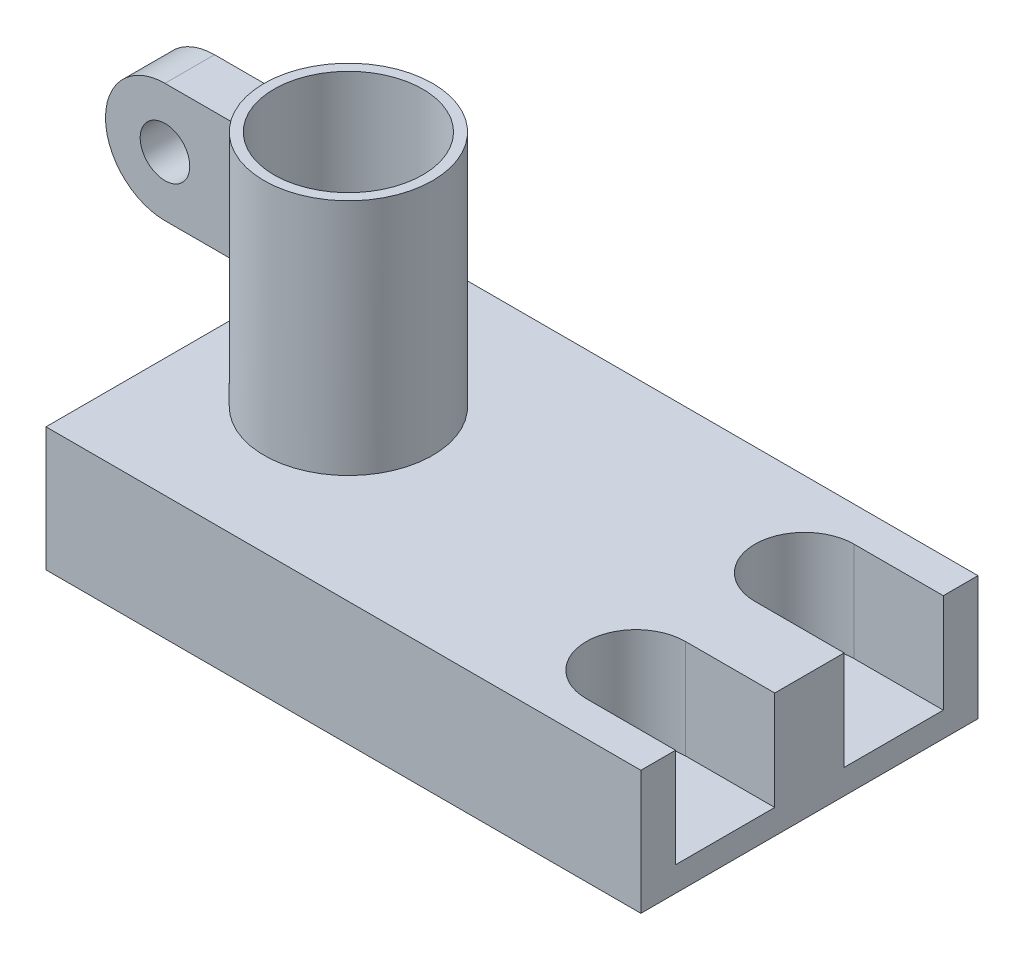
ISO-10303-21;
HEADER;
FILE_DESCRIPTION(('STEP AP214'),'2;1');
FILE_NAME('part.step','',(''),(''),'','','');
FILE_SCHEMA(('AUTOMOTIVE_DESIGN { 1 0 10303 214 1 1 1 1 }'));
ENDSEC;
DATA;
#1=APPLICATION_CONTEXT('core data for automotive mechanical design processes');
#2=APPLICATION_PROTOCOL_DEFINITION('international standard','automotive_design',2000,#1);
#3=PRODUCT_CONTEXT('',#1,'mechanical');
#4=PRODUCT('Part','Part','',(#3));
#5=PRODUCT_RELATED_PRODUCT_CATEGORY('part','',(#4));
#6=PRODUCT_DEFINITION_FORMATION('','',#4);
#7=PRODUCT_DEFINITION_CONTEXT('part definition',#1,'design');
#8=PRODUCT_DEFINITION('design','',#6,#7);
#9=PRODUCT_DEFINITION_SHAPE('','',#8);
#10=(LENGTH_UNIT() NAMED_UNIT(*) SI_UNIT(.MILLI.,.METRE.));
#11=(NAMED_UNIT(*) PLANE_ANGLE_UNIT() SI_UNIT($,.RADIAN.));
#12=(NAMED_UNIT(*) SI_UNIT($,.STERADIAN.) SOLID_ANGLE_UNIT());
#13=UNCERTAINTY_MEASURE_WITH_UNIT(LENGTH_MEASURE(1.E-05),#10,'distance_accuracy_value','');
#14=(GEOMETRIC_REPRESENTATION_CONTEXT(3) GLOBAL_UNCERTAINTY_ASSIGNED_CONTEXT((#13)) GLOBAL_UNIT_ASSIGNED_CONTEXT((#10,
#11,#12)) REPRESENTATION_CONTEXT('',''));
#15=CARTESIAN_POINT('',(0.,0.,0.));
#16=DIRECTION('',(0.,0.,1.));
#17=DIRECTION('',(1.,0.,0.));
#18=AXIS2_PLACEMENT_3D('',#15,#16,#17);
#19=CARTESIAN_POINT('',(60.,25.,34.));
#20=DIRECTION('',(-1.,0.,0.));
#21=DIRECTION('',(0.,0.,1.));
#22=AXIS2_PLACEMENT_3D('',#19,#20,#21);
#23=PLANE('',#22);
#24=DIRECTION('',(0.,0.,-1.));
#25=VECTOR('',#24,1.);
#26=CARTESIAN_POINT('',(60.,25.,34.));
#27=LINE('',#26,#25);
#28=CARTESIAN_POINT('',(60.,25.,-27.));
#29=VERTEX_POINT('',#28);
#30=CARTESIAN_POINT('',(60.,25.,-34.));
#31=VERTEX_POINT('',#30);
#32=EDGE_CURVE('E275',#29,#31,#27,.T.);
#33=ORIENTED_EDGE('',*,*,#32,.F.);
#34=DIRECTION('',(0.,1.,0.));
#35=VECTOR('',#34,1.);
#36=CARTESIAN_POINT('',(60.,5.,-27.));
#37=LINE('',#36,#35);
#38=CARTESIAN_POINT('',(60.,5.,-27.));
#39=VERTEX_POINT('',#38);
#40=EDGE_CURVE('E194',#39,#29,#37,.T.);
#41=ORIENTED_EDGE('',*,*,#40,.F.);
#42=DIRECTION('',(0.,0.,-1.));
#43=VECTOR('',#42,1.);
#44=CARTESIAN_POINT('',(60.,5.,-27.));
#45=LINE('',#44,#43);
#46=CARTESIAN_POINT('',(60.,5.,-6.99999999999999));
#47=VERTEX_POINT('',#46);
#48=EDGE_CURVE('E175',#47,#39,#45,.T.);
#49=ORIENTED_EDGE('',*,*,#48,.F.);
#50=DIRECTION('',(0.,1.,0.));
#51=VECTOR('',#50,1.);
#52=CARTESIAN_POINT('',(60.,5.,-6.99999999999999));
#53=LINE('',#52,#51);
#54=CARTESIAN_POINT('',(60.,25.,-6.99999999999999));
#55=VERTEX_POINT('',#54);
#56=EDGE_CURVE('E161',#47,#55,#53,.T.);
#57=ORIENTED_EDGE('',*,*,#56,.T.);
#58=CARTESIAN_POINT('',(60.,25.,7.00000000000001));
#59=VERTEX_POINT('',#58);
#60=EDGE_CURVE('E272',#59,#55,#27,.T.);
#61=ORIENTED_EDGE('',*,*,#60,.F.);
#62=DIRECTION('',(0.,1.,0.));
#63=VECTOR('',#62,1.);
#64=CARTESIAN_POINT('',(60.,5.,7.00000000000001));
#65=LINE('',#64,#63);
#66=CARTESIAN_POINT('',(60.,5.,7.00000000000001));
#67=VERTEX_POINT('',#66);
#68=EDGE_CURVE('E213',#67,#59,#65,.T.);
#69=ORIENTED_EDGE('',*,*,#68,.F.);
#70=DIRECTION('',(0.,0.,-1.));
#71=VECTOR('',#70,1.);
#72=CARTESIAN_POINT('',(60.,5.,7.00000000000001));
#73=LINE('',#72,#71);
#74=CARTESIAN_POINT('',(60.,5.,27.));
#75=VERTEX_POINT('',#74);
#76=EDGE_CURVE('E201',#75,#67,#73,.T.);
#77=ORIENTED_EDGE('',*,*,#76,.F.);
#78=DIRECTION('',(0.,1.,0.));
#79=VECTOR('',#78,1.);
#80=CARTESIAN_POINT('',(60.,5.,27.));
#81=LINE('',#80,#79);
#82=CARTESIAN_POINT('',(60.,25.,27.));
#83=VERTEX_POINT('',#82);
#84=EDGE_CURVE('E219',#75,#83,#81,.T.);
#85=ORIENTED_EDGE('',*,*,#84,.T.);
#86=CARTESIAN_POINT('',(60.,25.,34.));
#87=VERTEX_POINT('',#86);
#88=EDGE_CURVE('E270',#87,#83,#27,.T.);
#89=ORIENTED_EDGE('',*,*,#88,.F.);
#90=DIRECTION('',(0.,-1.,0.));
#91=VECTOR('',#90,1.);
#92=CARTESIAN_POINT('',(60.,25.,34.));
#93=LINE('',#92,#91);
#94=CARTESIAN_POINT('',(60.,0.,34.));
#95=VERTEX_POINT('',#94);
#96=EDGE_CURVE('E279',#87,#95,#93,.T.);
#97=ORIENTED_EDGE('',*,*,#96,.T.);
#98=DIRECTION('',(0.,0.,-1.));
#99=VECTOR('',#98,1.);
#100=CARTESIAN_POINT('',(60.,0.,34.));
#101=LINE('',#100,#99);
#102=CARTESIAN_POINT('',(60.,0.,-34.));
#103=VERTEX_POINT('',#102);
#104=EDGE_CURVE('E268',#95,#103,#101,.T.);
#105=ORIENTED_EDGE('',*,*,#104,.T.);
#106=DIRECTION('',(0.,-1.,0.));
#107=VECTOR('',#106,1.);
#108=CARTESIAN_POINT('',(60.,25.,-34.));
#109=LINE('',#108,#107);
#110=EDGE_CURVE('E294',#31,#103,#109,.T.);
#111=ORIENTED_EDGE('',*,*,#110,.F.);
#112=EDGE_LOOP('',(#33,#41,#49,#57,#61,#69,#77,#85,#89,#97,#105,#111));
#113=FACE_BOUND('',#112,.T.);
#114=ADVANCED_FACE('F44',(#113),#23,.F.);
#115=CARTESIAN_POINT('',(-60.,25.,-34.));
#116=DIRECTION('',(0.,0.,1.));
#117=DIRECTION('',(1.,0.,0.));
#118=AXIS2_PLACEMENT_3D('',#115,#116,#117);
#119=PLANE('',#118);
#120=DIRECTION('',(-1.,0.,0.));
#121=VECTOR('',#120,1.);
#122=CARTESIAN_POINT('',(-60.,0.,-34.));
#123=LINE('',#122,#121);
#124=CARTESIAN_POINT('',(-60.,0.,-34.));
#125=VERTEX_POINT('',#124);
#126=EDGE_CURVE('E283',#103,#125,#123,.T.);
#127=ORIENTED_EDGE('',*,*,#126,.T.);
#128=DIRECTION('',(0.,-1.,0.));
#129=VECTOR('',#128,1.);
#130=CARTESIAN_POINT('',(-60.,25.,-34.));
#131=LINE('',#130,#129);
#132=CARTESIAN_POINT('',(-60.,25.,-34.));
#133=VERTEX_POINT('',#132);
#134=EDGE_CURVE('E292',#133,#125,#131,.T.);
#135=ORIENTED_EDGE('',*,*,#134,.F.);
#136=DIRECTION('',(-1.,0.,0.));
#137=VECTOR('',#136,1.);
#138=CARTESIAN_POINT('',(-60.,25.,-34.));
#139=LINE('',#138,#137);
#140=EDGE_CURVE('E267',#31,#133,#139,.T.);
#141=ORIENTED_EDGE('',*,*,#140,.F.);
#142=ORIENTED_EDGE('',*,*,#110,.T.);
#143=EDGE_LOOP('',(#127,#135,#141,#142));
#144=FACE_BOUND('',#143,.T.);
#145=ADVANCED_FACE('F345',(#144),#119,.F.);
#146=CARTESIAN_POINT('',(-60.,25.,34.));
#147=DIRECTION('',(1.,0.,0.));
#148=DIRECTION('',(0.,0.,-1.));
#149=AXIS2_PLACEMENT_3D('',#146,#147,#148);
#150=PLANE('',#149);
#151=DIRECTION('',(0.,0.,1.));
#152=VECTOR('',#151,1.);
#153=CARTESIAN_POINT('',(-60.,0.,34.));
#154=LINE('',#153,#152);
#155=CARTESIAN_POINT('',(-60.,0.,34.));
#156=VERTEX_POINT('',#155);
#157=EDGE_CURVE('E282',#125,#156,#154,.T.);
#158=ORIENTED_EDGE('',*,*,#157,.T.);
#159=DIRECTION('',(0.,-1.,0.));
#160=VECTOR('',#159,1.);
#161=CARTESIAN_POINT('',(-60.,25.,34.));
#162=LINE('',#161,#160);
#163=CARTESIAN_POINT('',(-60.,25.,34.));
#164=VERTEX_POINT('',#163);
#165=EDGE_CURVE('E289',#164,#156,#162,.T.);
#166=ORIENTED_EDGE('',*,*,#165,.F.);
#167=DIRECTION('',(0.,0.,1.));
#168=VECTOR('',#167,1.);
#169=CARTESIAN_POINT('',(-60.,25.,34.));
#170=LINE('',#169,#168);
#171=EDGE_CURVE('E274',#133,#164,#170,.T.);
#172=ORIENTED_EDGE('',*,*,#171,.F.);
#173=ORIENTED_EDGE('',*,*,#134,.T.);
#174=EDGE_LOOP('',(#158,#166,#172,#173));
#175=FACE_BOUND('',#174,.T.);
#176=ADVANCED_FACE('F350',(#175),#150,.F.);
#177=CARTESIAN_POINT('',(-60.,25.,34.));
#178=DIRECTION('',(0.,0.,-1.));
#179=DIRECTION('',(-1.,0.,0.));
#180=AXIS2_PLACEMENT_3D('',#177,#178,#179);
#181=PLANE('',#180);
#182=DIRECTION('',(1.,0.,0.));
#183=VECTOR('',#182,1.);
#184=CARTESIAN_POINT('',(-60.,0.,34.));
#185=LINE('',#184,#183);
#186=EDGE_CURVE('E281',#156,#95,#185,.T.);
#187=ORIENTED_EDGE('',*,*,#186,.T.);
#188=ORIENTED_EDGE('',*,*,#96,.F.);
#189=DIRECTION('',(1.,0.,0.));
#190=VECTOR('',#189,1.);
#191=CARTESIAN_POINT('',(-60.,25.,34.));
#192=LINE('',#191,#190);
#193=EDGE_CURVE('E277',#164,#87,#192,.T.);
#194=ORIENTED_EDGE('',*,*,#193,.F.);
#195=ORIENTED_EDGE('',*,*,#165,.T.);
#196=EDGE_LOOP('',(#187,#188,#194,#195));
#197=FACE_BOUND('',#196,.T.);
#198=ADVANCED_FACE('F431',(#197),#181,.F.);
#199=CARTESIAN_POINT('',(0.,25.,0.));
#200=DIRECTION('',(0.,-1.,0.));
#201=DIRECTION('',(0.,0.,-1.));
#202=AXIS2_PLACEMENT_3D('',#199,#200,#201);
#203=PLANE('',#202);
#204=CARTESIAN_POINT('',(-33.,25.,0.));
#205=DIRECTION('',(0.,-1.,0.));
#206=DIRECTION('',(0.,0.,-1.));
#207=AXIS2_PLACEMENT_3D('',#204,#205,#206);
#208=CIRCLE('',#207,17.);
#209=CARTESIAN_POINT('',(-33.,25.,-17.));
#210=VERTEX_POINT('',#209);
#211=EDGE_CURVE('E296',#210,#210,#208,.F.);
#212=ORIENTED_EDGE('',*,*,#211,.F.);
#213=EDGE_LOOP('',(#212));
#214=FACE_BOUND('',#213,.T.);
#215=CARTESIAN_POINT('',(42.,25.,-17.));
#216=DIRECTION('',(0.,1.,0.));
#217=DIRECTION('',(0.,0.,1.));
#218=AXIS2_PLACEMENT_3D('',#215,#216,#217);
#219=CIRCLE('',#218,10.);
#220=CARTESIAN_POINT('',(42.,25.,-27.));
#221=VERTEX_POINT('',#220);
#222=CARTESIAN_POINT('',(42.,25.,-6.99999999999999));
#223=VERTEX_POINT('',#222);
#224=EDGE_CURVE('E58',#221,#223,#219,.T.);
#225=ORIENTED_EDGE('',*,*,#224,.F.);
#226=DIRECTION('',(-1.,0.,0.));
#227=VECTOR('',#226,1.);
#228=CARTESIAN_POINT('',(42.,25.,-27.));
#229=LINE('',#228,#227);
#230=EDGE_CURVE('E176',#29,#221,#229,.T.);
#231=ORIENTED_EDGE('',*,*,#230,.F.);
#232=ORIENTED_EDGE('',*,*,#32,.T.);
#233=ORIENTED_EDGE('',*,*,#140,.T.);
#234=ORIENTED_EDGE('',*,*,#171,.T.);
#235=ORIENTED_EDGE('',*,*,#193,.T.);
#236=ORIENTED_EDGE('',*,*,#88,.T.);
#237=DIRECTION('',(1.,0.,0.));
#238=VECTOR('',#237,1.);
#239=CARTESIAN_POINT('',(60.,25.,27.));
#240=LINE('',#239,#238);
#241=CARTESIAN_POINT('',(42.,25.,27.));
#242=VERTEX_POINT('',#241);
#243=EDGE_CURVE('E208',#242,#83,#240,.T.);
#244=ORIENTED_EDGE('',*,*,#243,.F.);
#245=CARTESIAN_POINT('',(42.,25.,17.));
#246=DIRECTION('',(0.,1.,0.));
#247=DIRECTION('',(0.,0.,1.));
#248=AXIS2_PLACEMENT_3D('',#245,#246,#247);
#249=CIRCLE('',#248,10.);
#250=CARTESIAN_POINT('',(42.,25.,7.00000000000001));
#251=VERTEX_POINT('',#250);
#252=EDGE_CURVE('E67',#251,#242,#249,.T.);
#253=ORIENTED_EDGE('',*,*,#252,.F.);
#254=DIRECTION('',(-1.,0.,0.));
#255=VECTOR('',#254,1.);
#256=CARTESIAN_POINT('',(42.,25.,7.00000000000001));
#257=LINE('',#256,#255);
#258=EDGE_CURVE('E196',#59,#251,#257,.T.);
#259=ORIENTED_EDGE('',*,*,#258,.F.);
#260=ORIENTED_EDGE('',*,*,#60,.T.);
#261=DIRECTION('',(1.,0.,0.));
#262=VECTOR('',#261,1.);
#263=CARTESIAN_POINT('',(60.,25.,-6.99999999999999));
#264=LINE('',#263,#262);
#265=EDGE_CURVE('E177',#223,#55,#264,.T.);
#266=ORIENTED_EDGE('',*,*,#265,.F.);
#267=EDGE_LOOP('',(#225,#231,#232,#233,#234,#235,#236,#244,#253,#259,#260,#266));
#268=FACE_BOUND('',#267,.T.);
#269=ADVANCED_FACE('F359',(#214,#268),#203,.F.);
#270=CARTESIAN_POINT('',(0.,0.,0.));
#271=DIRECTION('',(0.,-1.,0.));
#272=DIRECTION('',(0.,0.,-1.));
#273=AXIS2_PLACEMENT_3D('',#270,#271,#272);
#274=PLANE('',#273);
#275=CARTESIAN_POINT('',(42.,0.,-17.));
#276=DIRECTION('',(0.,-1.,0.));
#277=DIRECTION('',(0.,0.,-1.));
#278=AXIS2_PLACEMENT_3D('',#275,#276,#277);
#279=CIRCLE('',#278,4.00000000000001);
#280=CARTESIAN_POINT('',(42.,0.,-21.));
#281=VERTEX_POINT('',#280);
#282=EDGE_CURVE('E687',#281,#281,#279,.T.);
#283=ORIENTED_EDGE('',*,*,#282,.F.);
#284=EDGE_LOOP('',(#283));
#285=FACE_BOUND('',#284,.T.);
#286=CARTESIAN_POINT('',(42.,0.,17.));
#287=DIRECTION('',(0.,-1.,0.));
#288=DIRECTION('',(0.,0.,-1.));
#289=AXIS2_PLACEMENT_3D('',#286,#287,#288);
#290=CIRCLE('',#289,4.00000000000001);
#291=CARTESIAN_POINT('',(42.,0.,13.));
#292=VERTEX_POINT('',#291);
#293=EDGE_CURVE('E185',#292,#292,#290,.T.);
#294=ORIENTED_EDGE('',*,*,#293,.F.);
#295=EDGE_LOOP('',(#294));
#296=FACE_BOUND('',#295,.T.);
#297=CARTESIAN_POINT('',(-33.,0.,0.));
#298=DIRECTION('',(0.,1.,0.));
#299=DIRECTION('',(0.,0.,1.));
#300=AXIS2_PLACEMENT_3D('',#297,#298,#299);
#301=CIRCLE('',#300,15.);
#302=CARTESIAN_POINT('',(-33.,0.,15.));
#303=VERTEX_POINT('',#302);
#304=EDGE_CURVE('E221',#303,#303,#301,.T.);
#305=ORIENTED_EDGE('',*,*,#304,.T.);
#306=EDGE_LOOP('',(#305));
#307=FACE_BOUND('',#306,.T.);
#308=ORIENTED_EDGE('',*,*,#104,.F.);
#309=ORIENTED_EDGE('',*,*,#186,.F.);
#310=ORIENTED_EDGE('',*,*,#157,.F.);
#311=ORIENTED_EDGE('',*,*,#126,.F.);
#312=EDGE_LOOP('',(#308,#309,#310,#311));
#313=FACE_BOUND('',#312,.T.);
#314=ADVANCED_FACE('F429',(#285,#296,#307,#313),#274,.T.);
#315=CARTESIAN_POINT('',(-33.,73.,0.));
#316=DIRECTION('',(0.,-1.,0.));
#317=DIRECTION('',(0.,0.,-1.));
#318=AXIS2_PLACEMENT_3D('',#315,#316,#317);
#319=CYLINDRICAL_SURFACE('',#318,17.);
#320=CARTESIAN_POINT('',(-33.,68.,0.));
#321=DIRECTION('',(0.,-1.,0.));
#322=DIRECTION('',(0.,0.,-1.));
#323=AXIS2_PLACEMENT_3D('',#320,#321,#322);
#324=CIRCLE('',#323,17.);
#325=CARTESIAN_POINT('',(-49.2480768092719,68.,5.));
#326=VERTEX_POINT('',#325);
#327=CARTESIAN_POINT('',(-49.2480768092719,68.,-5.));
#328=VERTEX_POINT('',#327);
#329=EDGE_CURVE('E302',#326,#328,#324,.T.);
#330=ORIENTED_EDGE('',*,*,#329,.F.);
#331=DIRECTION('',(0.,-1.,0.));
#332=VECTOR('',#331,1.);
#333=CARTESIAN_POINT('',(-49.2480768092719,73.,5.));
#334=LINE('',#333,#332);
#335=CARTESIAN_POINT('',(-49.2480768092719,44.,5.));
#336=VERTEX_POINT('',#335);
#337=EDGE_CURVE('E11',#326,#336,#334,.T.);
#338=ORIENTED_EDGE('',*,*,#337,.T.);
#339=CARTESIAN_POINT('',(-33.,44.,0.));
#340=DIRECTION('',(0.,1.,0.));
#341=DIRECTION('',(0.,0.,1.));
#342=AXIS2_PLACEMENT_3D('',#339,#340,#341);
#343=CIRCLE('',#342,17.);
#344=CARTESIAN_POINT('',(-49.2480768092719,44.,-5.));
#345=VERTEX_POINT('',#344);
#346=EDGE_CURVE('E52',#345,#336,#343,.T.);
#347=ORIENTED_EDGE('',*,*,#346,.F.);
#348=DIRECTION('',(0.,-1.,0.));
#349=VECTOR('',#348,1.);
#350=CARTESIAN_POINT('',(-49.2480768092719,73.,-5.));
#351=LINE('',#350,#349);
#352=EDGE_CURVE('E301',#328,#345,#351,.T.);
#353=ORIENTED_EDGE('',*,*,#352,.F.);
#354=EDGE_LOOP('',(#330,#338,#347,#353));
#355=FACE_BOUND('',#354,.T.);
#356=CARTESIAN_POINT('',(-33.,73.,0.));
#357=DIRECTION('',(0.,1.,0.));
#358=DIRECTION('',(0.,0.,1.));
#359=AXIS2_PLACEMENT_3D('',#356,#357,#358);
#360=CIRCLE('',#359,17.);
#361=CARTESIAN_POINT('',(-33.,73.,17.));
#362=VERTEX_POINT('',#361);
#363=EDGE_CURVE('E262',#362,#362,#360,.T.);
#364=ORIENTED_EDGE('',*,*,#363,.F.);
#365=EDGE_LOOP('',(#364));
#366=FACE_BOUND('',#365,.T.);
#367=ORIENTED_EDGE('',*,*,#211,.T.);
#368=EDGE_LOOP('',(#367));
#369=FACE_BOUND('',#368,.T.);
#370=ADVANCED_FACE('F321',(#355,#366,#369),#319,.T.);
#371=CARTESIAN_POINT('',(-33.,73.,0.));
#372=DIRECTION('',(0.,1.,0.));
#373=DIRECTION('',(0.,0.,1.));
#374=AXIS2_PLACEMENT_3D('',#371,#372,#373);
#375=PLANE('',#374);
#376=CARTESIAN_POINT('',(-33.,73.,0.));
#377=DIRECTION('',(0.,1.,0.));
#378=DIRECTION('',(0.,0.,1.));
#379=AXIS2_PLACEMENT_3D('',#376,#377,#378);
#380=CIRCLE('',#379,15.);
#381=CARTESIAN_POINT('',(-33.,73.,15.));
#382=VERTEX_POINT('',#381);
#383=EDGE_CURVE('E232',#382,#382,#380,.T.);
#384=ORIENTED_EDGE('',*,*,#383,.F.);
#385=EDGE_LOOP('',(#384));
#386=FACE_BOUND('',#385,.T.);
#387=ORIENTED_EDGE('',*,*,#363,.T.);
#388=EDGE_LOOP('',(#387));
#389=FACE_BOUND('',#388,.T.);
#390=ADVANCED_FACE('F413',(#386,#389),#375,.T.);
#391=CARTESIAN_POINT('',(-65.,56.,5.));
#392=DIRECTION('',(0.,0.,1.));
#393=DIRECTION('',(1.,0.,0.));
#394=AXIS2_PLACEMENT_3D('',#391,#392,#393);
#395=PLANE('',#394);
#396=CARTESIAN_POINT('',(-65.,56.,5.));
#397=DIRECTION('',(0.,0.,1.));
#398=DIRECTION('',(1.,0.,0.));
#399=AXIS2_PLACEMENT_3D('',#396,#397,#398);
#400=CIRCLE('',#399,5.);
#401=CARTESIAN_POINT('',(-60.,56.,5.));
#402=VERTEX_POINT('',#401);
#403=EDGE_CURVE('E195',#402,#402,#400,.T.);
#404=ORIENTED_EDGE('',*,*,#403,.F.);
#405=EDGE_LOOP('',(#404));
#406=FACE_BOUND('',#405,.T.);
#407=ORIENTED_EDGE('',*,*,#337,.F.);
#408=DIRECTION('',(-1.,0.,0.));
#409=VECTOR('',#408,1.);
#410=CARTESIAN_POINT('',(-65.,68.,5.));
#411=LINE('',#410,#409);
#412=CARTESIAN_POINT('',(-65.,68.,5.));
#413=VERTEX_POINT('',#412);
#414=EDGE_CURVE('E248',#326,#413,#411,.T.);
#415=ORIENTED_EDGE('',*,*,#414,.T.);
#416=CARTESIAN_POINT('',(-65.,56.,5.));
#417=DIRECTION('',(0.,0.,1.));
#418=DIRECTION('',(1.,0.,0.));
#419=AXIS2_PLACEMENT_3D('',#416,#417,#418);
#420=CIRCLE('',#419,12.);
#421=CARTESIAN_POINT('',(-65.,44.,5.));
#422=VERTEX_POINT('',#421);
#423=EDGE_CURVE('E245',#413,#422,#420,.T.);
#424=ORIENTED_EDGE('',*,*,#423,.T.);
#425=DIRECTION('',(1.,0.,0.));
#426=VECTOR('',#425,1.);
#427=CARTESIAN_POINT('',(-48.8983725449501,44.,5.));
#428=LINE('',#427,#426);
#429=EDGE_CURVE('E244',#422,#336,#428,.T.);
#430=ORIENTED_EDGE('',*,*,#429,.T.);
#431=EDGE_LOOP('',(#407,#415,#424,#430));
#432=FACE_BOUND('',#431,.T.);
#433=ADVANCED_FACE('F312',(#406,#432),#395,.T.);
#434=CARTESIAN_POINT('',(-65.,56.,-5.));
#435=DIRECTION('',(0.,0.,1.));
#436=DIRECTION('',(1.,0.,0.));
#437=AXIS2_PLACEMENT_3D('',#434,#435,#436);
#438=PLANE('',#437);
#439=CARTESIAN_POINT('',(-65.,56.,-5.));
#440=DIRECTION('',(0.,0.,1.));
#441=DIRECTION('',(1.,0.,0.));
#442=AXIS2_PLACEMENT_3D('',#439,#440,#441);
#443=CIRCLE('',#442,5.);
#444=CARTESIAN_POINT('',(-60.,56.,-5.));
#445=VERTEX_POINT('',#444);
#446=EDGE_CURVE('E48',#445,#445,#443,.T.);
#447=ORIENTED_EDGE('',*,*,#446,.T.);
#448=EDGE_LOOP('',(#447));
#449=FACE_BOUND('',#448,.T.);
#450=DIRECTION('',(-1.,0.,0.));
#451=VECTOR('',#450,1.);
#452=CARTESIAN_POINT('',(-65.,68.,-5.));
#453=LINE('',#452,#451);
#454=CARTESIAN_POINT('',(-65.,68.,-5.));
#455=VERTEX_POINT('',#454);
#456=EDGE_CURVE('E246',#328,#455,#453,.T.);
#457=ORIENTED_EDGE('',*,*,#456,.F.);
#458=ORIENTED_EDGE('',*,*,#352,.T.);
#459=DIRECTION('',(1.,0.,0.));
#460=VECTOR('',#459,1.);
#461=CARTESIAN_POINT('',(-48.8983725449501,44.,-5.));
#462=LINE('',#461,#460);
#463=CARTESIAN_POINT('',(-65.,44.,-5.));
#464=VERTEX_POINT('',#463);
#465=EDGE_CURVE('E251',#464,#345,#462,.T.);
#466=ORIENTED_EDGE('',*,*,#465,.F.);
#467=CARTESIAN_POINT('',(-65.,56.,-5.));
#468=DIRECTION('',(0.,0.,1.));
#469=DIRECTION('',(1.,0.,0.));
#470=AXIS2_PLACEMENT_3D('',#467,#468,#469);
#471=CIRCLE('',#470,12.);
#472=EDGE_CURVE('E237',#455,#464,#471,.T.);
#473=ORIENTED_EDGE('',*,*,#472,.F.);
#474=EDGE_LOOP('',(#457,#458,#466,#473));
#475=FACE_BOUND('',#474,.T.);
#476=ADVANCED_FACE('F324',(#449,#475),#438,.F.);
#477=CARTESIAN_POINT('',(-65.,56.,5.));
#478=DIRECTION('',(0.,0.,-1.));
#479=DIRECTION('',(-1.,0.,0.));
#480=AXIS2_PLACEMENT_3D('',#477,#478,#479);
#481=CYLINDRICAL_SURFACE('',#480,12.);
#482=ORIENTED_EDGE('',*,*,#472,.T.);
#483=DIRECTION('',(0.,0.,-1.));
#484=VECTOR('',#483,1.);
#485=CARTESIAN_POINT('',(-65.,44.,5.));
#486=LINE('',#485,#484);
#487=EDGE_CURVE('E258',#422,#464,#486,.T.);
#488=ORIENTED_EDGE('',*,*,#487,.F.);
#489=ORIENTED_EDGE('',*,*,#423,.F.);
#490=DIRECTION('',(0.,0.,-1.));
#491=VECTOR('',#490,1.);
#492=CARTESIAN_POINT('',(-65.,68.,5.));
#493=LINE('',#492,#491);
#494=EDGE_CURVE('E252',#413,#455,#493,.T.);
#495=ORIENTED_EDGE('',*,*,#494,.T.);
#496=EDGE_LOOP('',(#482,#488,#489,#495));
#497=FACE_BOUND('',#496,.T.);
#498=ADVANCED_FACE('F316',(#497),#481,.T.);
#499=CARTESIAN_POINT('',(-48.8983725449501,44.,5.));
#500=DIRECTION('',(0.,1.,0.));
#501=DIRECTION('',(0.,0.,1.));
#502=AXIS2_PLACEMENT_3D('',#499,#500,#501);
#503=PLANE('',#502);
#504=ORIENTED_EDGE('',*,*,#465,.T.);
#505=ORIENTED_EDGE('',*,*,#346,.T.);
#506=ORIENTED_EDGE('',*,*,#429,.F.);
#507=ORIENTED_EDGE('',*,*,#487,.T.);
#508=EDGE_LOOP('',(#504,#505,#506,#507));
#509=FACE_BOUND('',#508,.T.);
#510=ADVANCED_FACE('F307',(#509),#503,.F.);
#511=CARTESIAN_POINT('',(-65.,68.,5.));
#512=DIRECTION('',(0.,-1.,0.));
#513=DIRECTION('',(0.,0.,-1.));
#514=AXIS2_PLACEMENT_3D('',#511,#512,#513);
#515=PLANE('',#514);
#516=ORIENTED_EDGE('',*,*,#414,.F.);
#517=ORIENTED_EDGE('',*,*,#329,.T.);
#518=ORIENTED_EDGE('',*,*,#456,.T.);
#519=ORIENTED_EDGE('',*,*,#494,.F.);
#520=EDGE_LOOP('',(#516,#517,#518,#519));
#521=FACE_BOUND('',#520,.T.);
#522=ADVANCED_FACE('F329',(#521),#515,.F.);
#523=CARTESIAN_POINT('',(-33.,40.,0.));
#524=DIRECTION('',(0.,1.,0.));
#525=DIRECTION('',(0.,0.,1.));
#526=AXIS2_PLACEMENT_3D('',#523,#524,#525);
#527=CYLINDRICAL_SURFACE('',#526,15.);
#528=CARTESIAN_POINT('',(-33.,40.,0.));
#529=DIRECTION('',(0.,1.,0.));
#530=DIRECTION('',(0.,0.,1.));
#531=AXIS2_PLACEMENT_3D('',#528,#529,#530);
#532=CIRCLE('',#531,15.);
#533=CARTESIAN_POINT('',(-33.,40.,15.));
#534=VERTEX_POINT('',#533);
#535=EDGE_CURVE('E236',#534,#534,#532,.T.);
#536=ORIENTED_EDGE('',*,*,#535,.F.);
#537=EDGE_LOOP('',(#536));
#538=FACE_BOUND('',#537,.T.);
#539=ORIENTED_EDGE('',*,*,#383,.T.);
#540=EDGE_LOOP('',(#539));
#541=FACE_BOUND('',#540,.T.);
#542=ADVANCED_FACE('F330',(#538,#541),#527,.F.);
#543=CARTESIAN_POINT('',(-33.,40.,0.));
#544=DIRECTION('',(0.,1.,0.));
#545=DIRECTION('',(0.,0.,1.));
#546=AXIS2_PLACEMENT_3D('',#543,#544,#545);
#547=PLANE('',#546);
#548=CARTESIAN_POINT('',(-33.,40.,0.));
#549=DIRECTION('',(0.,1.,0.));
#550=DIRECTION('',(0.,0.,1.));
#551=AXIS2_PLACEMENT_3D('',#548,#549,#550);
#552=CIRCLE('',#551,9.);
#553=CARTESIAN_POINT('',(-33.,40.,9.));
#554=VERTEX_POINT('',#553);
#555=EDGE_CURVE('E235',#554,#554,#552,.T.);
#556=ORIENTED_EDGE('',*,*,#555,.F.);
#557=EDGE_LOOP('',(#556));
#558=FACE_BOUND('',#557,.T.);
#559=ORIENTED_EDGE('',*,*,#535,.T.);
#560=EDGE_LOOP('',(#559));
#561=FACE_BOUND('',#560,.T.);
#562=ADVANCED_FACE('F337',(#558,#561),#547,.T.);
#563=CARTESIAN_POINT('',(-33.,30.,0.));
#564=DIRECTION('',(0.,1.,0.));
#565=DIRECTION('',(0.,0.,1.));
#566=AXIS2_PLACEMENT_3D('',#563,#564,#565);
#567=CYLINDRICAL_SURFACE('',#566,9.);
#568=CARTESIAN_POINT('',(-33.,30.,0.));
#569=DIRECTION('',(0.,1.,0.));
#570=DIRECTION('',(0.,0.,1.));
#571=AXIS2_PLACEMENT_3D('',#568,#569,#570);
#572=CIRCLE('',#571,9.);
#573=CARTESIAN_POINT('',(-33.,30.,9.));
#574=VERTEX_POINT('',#573);
#575=EDGE_CURVE('E228',#574,#574,#572,.T.);
#576=ORIENTED_EDGE('',*,*,#575,.F.);
#577=EDGE_LOOP('',(#576));
#578=FACE_BOUND('',#577,.T.);
#579=ORIENTED_EDGE('',*,*,#555,.T.);
#580=EDGE_LOOP('',(#579));
#581=FACE_BOUND('',#580,.T.);
#582=ADVANCED_FACE('F405',(#578,#581),#567,.F.);
#583=CARTESIAN_POINT('',(-33.,0.,0.));
#584=DIRECTION('',(0.,1.,0.));
#585=DIRECTION('',(0.,0.,1.));
#586=AXIS2_PLACEMENT_3D('',#583,#584,#585);
#587=CYLINDRICAL_SURFACE('',#586,15.);
#588=ORIENTED_EDGE('',*,*,#304,.F.);
#589=EDGE_LOOP('',(#588));
#590=FACE_BOUND('',#589,.T.);
#591=CARTESIAN_POINT('',(-33.,30.,0.));
#592=DIRECTION('',(0.,1.,0.));
#593=DIRECTION('',(0.,0.,1.));
#594=AXIS2_PLACEMENT_3D('',#591,#592,#593);
#595=CIRCLE('',#594,15.);
#596=CARTESIAN_POINT('',(-33.,30.,15.));
#597=VERTEX_POINT('',#596);
#598=EDGE_CURVE('E227',#597,#597,#595,.T.);
#599=ORIENTED_EDGE('',*,*,#598,.T.);
#600=EDGE_LOOP('',(#599));
#601=FACE_BOUND('',#600,.T.);
#602=ADVANCED_FACE('F396',(#590,#601),#587,.F.);
#603=CARTESIAN_POINT('',(-33.,30.,0.));
#604=DIRECTION('',(0.,1.,0.));
#605=DIRECTION('',(0.,0.,1.));
#606=AXIS2_PLACEMENT_3D('',#603,#604,#605);
#607=PLANE('',#606);
#608=ORIENTED_EDGE('',*,*,#575,.T.);
#609=EDGE_LOOP('',(#608));
#610=FACE_BOUND('',#609,.T.);
#611=ORIENTED_EDGE('',*,*,#598,.F.);
#612=EDGE_LOOP('',(#611));
#613=FACE_BOUND('',#612,.T.);
#614=ADVANCED_FACE('F395',(#610,#613),#607,.F.);
#615=CARTESIAN_POINT('',(-65.,56.,-20.));
#616=DIRECTION('',(0.,0.,1.));
#617=DIRECTION('',(1.,0.,0.));
#618=AXIS2_PLACEMENT_3D('',#615,#616,#617);
#619=CYLINDRICAL_SURFACE('',#618,5.);
#620=ORIENTED_EDGE('',*,*,#403,.T.);
#621=EDGE_LOOP('',(#620));
#622=FACE_BOUND('',#621,.T.);
#623=ORIENTED_EDGE('',*,*,#446,.F.);
#624=EDGE_LOOP('',(#623));
#625=FACE_BOUND('',#624,.T.);
#626=ADVANCED_FACE('F393',(#622,#625),#619,.F.);
#627=CARTESIAN_POINT('',(42.,5.,17.));
#628=DIRECTION('',(0.,1.,0.));
#629=DIRECTION('',(0.,0.,1.));
#630=AXIS2_PLACEMENT_3D('',#627,#628,#629);
#631=CYLINDRICAL_SURFACE('',#630,10.);
#632=ORIENTED_EDGE('',*,*,#252,.T.);
#633=DIRECTION('',(0.,1.,0.));
#634=VECTOR('',#633,1.);
#635=CARTESIAN_POINT('',(42.,5.,27.));
#636=LINE('',#635,#634);
#637=CARTESIAN_POINT('',(42.,5.,27.));
#638=VERTEX_POINT('',#637);
#639=EDGE_CURVE('E206',#638,#242,#636,.T.);
#640=ORIENTED_EDGE('',*,*,#639,.F.);
#641=CARTESIAN_POINT('',(42.,5.,17.));
#642=DIRECTION('',(0.,1.,0.));
#643=DIRECTION('',(0.,0.,1.));
#644=AXIS2_PLACEMENT_3D('',#641,#642,#643);
#645=CIRCLE('',#644,10.);
#646=CARTESIAN_POINT('',(42.,5.,7.00000000000001));
#647=VERTEX_POINT('',#646);
#648=EDGE_CURVE('E198',#647,#638,#645,.T.);
#649=ORIENTED_EDGE('',*,*,#648,.F.);
#650=DIRECTION('',(0.,1.,0.));
#651=VECTOR('',#650,1.);
#652=CARTESIAN_POINT('',(42.,5.,7.00000000000001));
#653=LINE('',#652,#651);
#654=EDGE_CURVE('E189',#647,#251,#653,.T.);
#655=ORIENTED_EDGE('',*,*,#654,.T.);
#656=EDGE_LOOP('',(#632,#640,#649,#655));
#657=FACE_BOUND('',#656,.T.);
#658=ADVANCED_FACE('F381',(#657),#631,.F.);
#659=CARTESIAN_POINT('',(42.,5.,7.00000000000001));
#660=DIRECTION('',(0.,0.,-1.));
#661=DIRECTION('',(-1.,0.,0.));
#662=AXIS2_PLACEMENT_3D('',#659,#660,#661);
#663=PLANE('',#662);
#664=ORIENTED_EDGE('',*,*,#258,.T.);
#665=ORIENTED_EDGE('',*,*,#654,.F.);
#666=DIRECTION('',(-1.,0.,0.));
#667=VECTOR('',#666,1.);
#668=CARTESIAN_POINT('',(42.,5.,7.00000000000001));
#669=LINE('',#668,#667);
#670=EDGE_CURVE('E202',#67,#647,#669,.T.);
#671=ORIENTED_EDGE('',*,*,#670,.F.);
#672=ORIENTED_EDGE('',*,*,#68,.T.);
#673=EDGE_LOOP('',(#664,#665,#671,#672));
#674=FACE_BOUND('',#673,.T.);
#675=ADVANCED_FACE('F382',(#674),#663,.F.);
#676=CARTESIAN_POINT('',(60.,5.,27.));
#677=DIRECTION('',(0.,0.,1.));
#678=DIRECTION('',(1.,0.,0.));
#679=AXIS2_PLACEMENT_3D('',#676,#677,#678);
#680=PLANE('',#679);
#681=ORIENTED_EDGE('',*,*,#243,.T.);
#682=ORIENTED_EDGE('',*,*,#84,.F.);
#683=DIRECTION('',(1.,0.,0.));
#684=VECTOR('',#683,1.);
#685=CARTESIAN_POINT('',(60.,5.,27.));
#686=LINE('',#685,#684);
#687=EDGE_CURVE('E200',#638,#75,#686,.T.);
#688=ORIENTED_EDGE('',*,*,#687,.F.);
#689=ORIENTED_EDGE('',*,*,#639,.T.);
#690=EDGE_LOOP('',(#681,#682,#688,#689));
#691=FACE_BOUND('',#690,.T.);
#692=ADVANCED_FACE('F378',(#691),#680,.F.);
#693=CARTESIAN_POINT('',(42.,5.,17.));
#694=DIRECTION('',(0.,1.,0.));
#695=DIRECTION('',(0.,0.,1.));
#696=AXIS2_PLACEMENT_3D('',#693,#694,#695);
#697=PLANE('',#696);
#698=CARTESIAN_POINT('',(42.,5.,17.));
#699=DIRECTION('',(0.,1.,0.));
#700=DIRECTION('',(0.,0.,1.));
#701=AXIS2_PLACEMENT_3D('',#698,#699,#700);
#702=CIRCLE('',#701,4.00000000000001);
#703=CARTESIAN_POINT('',(42.,5.,21.));
#704=VERTEX_POINT('',#703);
#705=EDGE_CURVE('E688',#704,#704,#702,.T.);
#706=ORIENTED_EDGE('',*,*,#705,.F.);
#707=EDGE_LOOP('',(#706));
#708=FACE_BOUND('',#707,.T.);
#709=ORIENTED_EDGE('',*,*,#648,.T.);
#710=ORIENTED_EDGE('',*,*,#687,.T.);
#711=ORIENTED_EDGE('',*,*,#76,.T.);
#712=ORIENTED_EDGE('',*,*,#670,.T.);
#713=EDGE_LOOP('',(#709,#710,#711,#712));
#714=FACE_BOUND('',#713,.T.);
#715=ADVANCED_FACE('F375',(#708,#714),#697,.T.);
#716=CARTESIAN_POINT('',(42.,5.,-17.));
#717=DIRECTION('',(0.,1.,0.));
#718=DIRECTION('',(0.,0.,1.));
#719=AXIS2_PLACEMENT_3D('',#716,#717,#718);
#720=CYLINDRICAL_SURFACE('',#719,10.);
#721=ORIENTED_EDGE('',*,*,#224,.T.);
#722=DIRECTION('',(0.,1.,0.));
#723=VECTOR('',#722,1.);
#724=CARTESIAN_POINT('',(42.,5.,-6.99999999999999));
#725=LINE('',#724,#723);
#726=CARTESIAN_POINT('',(42.,5.,-6.99999999999999));
#727=VERTEX_POINT('',#726);
#728=EDGE_CURVE('E151',#727,#223,#725,.T.);
#729=ORIENTED_EDGE('',*,*,#728,.F.);
#730=CARTESIAN_POINT('',(42.,5.,-17.));
#731=DIRECTION('',(0.,1.,0.));
#732=DIRECTION('',(0.,0.,1.));
#733=AXIS2_PLACEMENT_3D('',#730,#731,#732);
#734=CIRCLE('',#733,10.);
#735=CARTESIAN_POINT('',(42.,5.,-27.));
#736=VERTEX_POINT('',#735);
#737=EDGE_CURVE('E159',#736,#727,#734,.T.);
#738=ORIENTED_EDGE('',*,*,#737,.F.);
#739=DIRECTION('',(0.,1.,0.));
#740=VECTOR('',#739,1.);
#741=CARTESIAN_POINT('',(42.,5.,-27.));
#742=LINE('',#741,#740);
#743=EDGE_CURVE('E188',#736,#221,#742,.T.);
#744=ORIENTED_EDGE('',*,*,#743,.T.);
#745=EDGE_LOOP('',(#721,#729,#738,#744));
#746=FACE_BOUND('',#745,.T.);
#747=ADVANCED_FACE('F160',(#746),#720,.F.);
#748=CARTESIAN_POINT('',(42.,5.,-27.));
#749=DIRECTION('',(0.,0.,-1.));
#750=DIRECTION('',(-1.,0.,0.));
#751=AXIS2_PLACEMENT_3D('',#748,#749,#750);
#752=PLANE('',#751);
#753=ORIENTED_EDGE('',*,*,#230,.T.);
#754=ORIENTED_EDGE('',*,*,#743,.F.);
#755=DIRECTION('',(-1.,0.,0.));
#756=VECTOR('',#755,1.);
#757=CARTESIAN_POINT('',(42.,5.,-27.));
#758=LINE('',#757,#756);
#759=EDGE_CURVE('E165',#39,#736,#758,.T.);
#760=ORIENTED_EDGE('',*,*,#759,.F.);
#761=ORIENTED_EDGE('',*,*,#40,.T.);
#762=EDGE_LOOP('',(#753,#754,#760,#761));
#763=FACE_BOUND('',#762,.T.);
#764=ADVANCED_FACE('F364',(#763),#752,.F.);
#765=CARTESIAN_POINT('',(60.,5.,-6.99999999999999));
#766=DIRECTION('',(0.,0.,1.));
#767=DIRECTION('',(1.,0.,0.));
#768=AXIS2_PLACEMENT_3D('',#765,#766,#767);
#769=PLANE('',#768);
#770=ORIENTED_EDGE('',*,*,#265,.T.);
#771=ORIENTED_EDGE('',*,*,#56,.F.);
#772=DIRECTION('',(1.,0.,0.));
#773=VECTOR('',#772,1.);
#774=CARTESIAN_POINT('',(60.,5.,-6.99999999999999));
#775=LINE('',#774,#773);
#776=EDGE_CURVE('E170',#727,#47,#775,.T.);
#777=ORIENTED_EDGE('',*,*,#776,.F.);
#778=ORIENTED_EDGE('',*,*,#728,.T.);
#779=EDGE_LOOP('',(#770,#771,#777,#778));
#780=FACE_BOUND('',#779,.T.);
#781=ADVANCED_FACE('F166',(#780),#769,.F.);
#782=CARTESIAN_POINT('',(42.,5.,-17.));
#783=DIRECTION('',(0.,1.,0.));
#784=DIRECTION('',(0.,0.,1.));
#785=AXIS2_PLACEMENT_3D('',#782,#783,#784);
#786=PLANE('',#785);
#787=CARTESIAN_POINT('',(42.,5.,-17.));
#788=DIRECTION('',(0.,1.,0.));
#789=DIRECTION('',(0.,0.,1.));
#790=AXIS2_PLACEMENT_3D('',#787,#788,#789);
#791=CIRCLE('',#790,4.00000000000001);
#792=CARTESIAN_POINT('',(42.,5.,-13.));
#793=VERTEX_POINT('',#792);
#794=EDGE_CURVE('E690',#793,#793,#791,.T.);
#795=ORIENTED_EDGE('',*,*,#794,.F.);
#796=EDGE_LOOP('',(#795));
#797=FACE_BOUND('',#796,.T.);
#798=ORIENTED_EDGE('',*,*,#737,.T.);
#799=ORIENTED_EDGE('',*,*,#776,.T.);
#800=ORIENTED_EDGE('',*,*,#48,.T.);
#801=ORIENTED_EDGE('',*,*,#759,.T.);
#802=EDGE_LOOP('',(#798,#799,#800,#801));
#803=FACE_BOUND('',#802,.T.);
#804=ADVANCED_FACE('F172',(#797,#803),#786,.T.);
#805=CARTESIAN_POINT('',(42.,-15.,-17.));
#806=DIRECTION('',(0.,1.,0.));
#807=DIRECTION('',(0.,0.,1.));
#808=AXIS2_PLACEMENT_3D('',#805,#806,#807);
#809=CYLINDRICAL_SURFACE('',#808,4.00000000000001);
#810=ORIENTED_EDGE('',*,*,#282,.T.);
#811=EDGE_LOOP('',(#810));
#812=FACE_BOUND('',#811,.T.);
#813=ORIENTED_EDGE('',*,*,#794,.T.);
#814=EDGE_LOOP('',(#813));
#815=FACE_BOUND('',#814,.T.);
#816=ADVANCED_FACE('F615',(#812,#815),#809,.F.);
#817=CARTESIAN_POINT('',(42.,-15.,17.));
#818=DIRECTION('',(0.,1.,0.));
#819=DIRECTION('',(0.,0.,1.));
#820=AXIS2_PLACEMENT_3D('',#817,#818,#819);
#821=CYLINDRICAL_SURFACE('',#820,4.00000000000001);
#822=ORIENTED_EDGE('',*,*,#293,.T.);
#823=EDGE_LOOP('',(#822));
#824=FACE_BOUND('',#823,.T.);
#825=ORIENTED_EDGE('',*,*,#705,.T.);
#826=EDGE_LOOP('',(#825));
#827=FACE_BOUND('',#826,.T.);
#828=ADVANCED_FACE('F625',(#824,#827),#821,.F.);
#829=CLOSED_SHELL('',(#114,#145,#176,#198,#269,#314,#370,#390,#433,#476,#498,#510,#522,#542,
#562,#582,#602,#614,#626,#658,#675,#692,#715,#747,#764,#781,#804,#816,#828));
#830=MANIFOLD_SOLID_BREP('B2',#829);
#831=ADVANCED_BREP_SHAPE_REPRESENTATION('',(#18,#830),#14);
#832=SHAPE_DEFINITION_REPRESENTATION(#9,#831);
ENDSEC;
END-ISO-10303-21;
